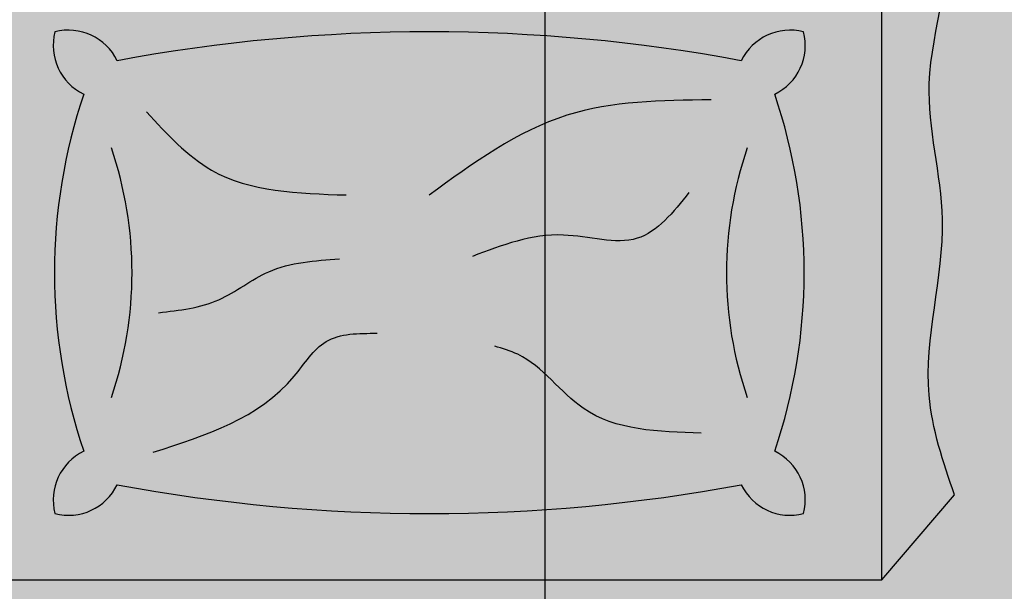
# Model space of a CAD drawing. Units: inches. Extents: x 1704 to 6393, y -157 to 1172.
# Tile 34 of 122: x 2529 to 2563, y 112 to 131. Entities that reach past the tile are written whole.
import ezdxf

# ---------------------------------------------------------------- set-up
doc = ezdxf.new("R2010")
doc.units = ezdxf.units.IN
doc.header["$MEASUREMENT"] = 0
for name, color, linetype, lineweight in [('A-ANNO-DIMS', 7, 'Continuous', 13), ('A-FURN', 8, 'Continuous', 18), ('estofado', 7, 'Continuous', 25)]:
    doc.layers.add(name, color=color, linetype=linetype, lineweight=lineweight)
doc.layers.add('A-FLOR-PATT', color=7, linetype='Continuous', lineweight=13, true_color=0xf2f2f2)
doc.styles.get("Standard").update_dxf_attribs({"font": 'arial.ttf'})
doc.dimstyles.get("Standard").update_dxf_attribs({"dimtxt": 6, "dimasz": 2, "dimexe": 0.18, "dimexo": 0.0625, "dimgap": 0.09, "dimtad": 0, "dimtih": 1, "dimtoh": 1, "dimdec": 1, "dimzin": 0, "dimdsep": 46, "dimlunit": 3, "dimtxsty": 'Standard', "dimblk": 'ARCHTICK', "dimcen": 0.09, "dimadec": 0, "dimazin": 0, "dimtfac": 1, "dimtdec": 1, "dimtofl": 0, "dimtmove": 0, "dimatfit": 3, "dimfxl": 1, "dimtolj": 1, "dimtzin": 0, "dimarcsym": 0})

# ---------------------------------------------------------------- blocks, each defined once
blk = doc.blocks.new('Cama Box Regencia LOLA')
at = {"layer": 'estofado', "ltscale": 0.2}
h = blk.add_hatch(color=256, dxfattribs=at)
h.dxf.hatch_style = 1
h.set_gradient(color1=(240, 232, 219), color2=(213, 190, 154), one_color=1, tint=0.7200000286102295)
edge = h.paths.add_edge_path()
edge.add_line((-0.8000000000000682, -0.1548023628405417), (-0.863597199697665, -0.2293271111754507))
edge.add_spline(control_points=[(-0.8635971996977787, -0.2293271111754507), (-0.8537222782123308, -0.258285373872468), (-0.8269013755602826, -0.3369378214810581), (-0.8674912876567759, -0.4595932758330151), (-0.8253488717912205, -0.6001498518888299), (-0.8771423076391329, -0.7139760714239288), (-0.8243323781925938, -0.8129899320257435), (-0.885044987287756, -0.8716602542656914), (-0.879518062107536, -0.9542863467743244), (-0.8339551707063037, -1.008464155856984), (-0.8245672924600739, -1.059984630119799), (-0.8208601923470268, -1.104655887174089), (-0.8073908324747662, -1.131238421004809), (-0.7999999999999546, -1.145824641594799)], knot_values=[0, 0, 0, 0, 0.0901802310564388, 0.2449351320798513, 0.3646438241986237, 0.5132330690395209, 0.5950634960661151, 0.646820388242338, 0.740988272125753, 0.8098674202588053, 0.8551784313864677, 0.8950360916221496, 0.9434986994854018, 0.9434986994854018, 0.9434986994854018, 0.9434986994854018], degree=3, periodic=0)
edge.add_line((-0.7999999999999546, -1.145824641594856), (-0.7999999999999546, -0.9571831923306604))
edge.add_spline(control_points=[(-0.8000000000001818, -0.9571831923294098), (-0.8003674620557603, -0.9560020588672273), (-0.8014778173377408, -0.9524330433489467), (-0.799534669348418, -0.9460450666617248), (-0.7963405736333016, -0.9382358308520792), (-0.7944188048602429, -0.9289040147384638), (-0.7953122817383474, -0.9190683391483389), (-0.7985341887020923, -0.9137677522519994), (-0.7999999999999546, -0.911356242470788)], knot_values=[0, 0, 0, 0, 0.0036609130031785, 0.0110621328900358, 0.0190316076023675, 0.0292873612819121, 0.0393286152452009, 0.0477100398955968, 0.0477100398955968, 0.0477100398955968, 0.0477100398955968], degree=3, periodic=0)
edge.add_line((-0.8000000000000682, -0.9113562424705037), (-0.7999999999999546, -0.8573491405791173))
edge.add_spline(control_points=[(-0.7999999999999546, -0.8573491405791173), (-0.8011509914009592, -0.8570771933481751), (-0.804102924754261, -0.8563797336621519), (-0.8039036519178353, -0.8498286502876908), (-0.8010279369466388, -0.8413595542568258), (-0.805623441450507, -0.8302818657685406), (-0.801318481758244, -0.8238273834048186), (-0.7999999999999546, -0.8218505664625013)], knot_values=[0, 0, 0, 0, 0.0032305881034183, 0.0082854491905874, 0.015951437769388, 0.0315866871777379, 0.0384893971878813, 0.0384893971878813, 0.0384893971878813, 0.0384893971878813], degree=3, periodic=0)
edge.add_line((-0.7999999999999546, -0.821850566462558), (-0.7999999999999546, -0.7800193173444541))
edge.add_spline(control_points=[(-0.7999999999999546, -0.7800193173443404), (-0.7985416092056994, -0.7788853679199974), (-0.7956241855360986, -0.7766169698310819), (-0.7929439183725436, -0.7707329795046576), (-0.7969680334608711, -0.7644035258254576), (-0.7912681985083055, -0.7566015403456845), (-0.7963938877088595, -0.7483952775559715), (-0.798936373489596, -0.7431699116222604), (-0.799999999999841, -0.7409839258539251)], knot_values=[0, 0, 0, 0, 0.0055481279082489, 0.0110986984731684, 0.0174746050947868, 0.0251556172852474, 0.035519246289823, 0.0429729849735991, 0.0429729849735991, 0.0429729849735991, 0.0429729849735991], degree=3, periodic=0)
edge.add_line((-0.7999999999999546, -0.740983925853584), (-0.8000000000000682, -0.1548023628405417))
h = blk.add_hatch(color=256, dxfattribs=at)
h.dxf.hatch_style = 1
h.set_gradient(color1=(240, 232, 219), color2=(213, 190, 154), one_color=1, tint=0.7200000286102295, name='CURVED')
edge = h.paths.add_edge_path()
edge.add_spline(control_points=[(0.343533776195045, -0.8455058148597345), (0.2879313990920309, -0.8167160606696484), (0.2054770794474052, -0.7744470032542381), (0.0954193394759386, -0.7742416952675626), (-0.0885363502328574, -0.7276964167006668), (0.2428192566063672, -0.7672518992321216), (0.345087521536243, -0.8076697826234067), (0.3825206986321063, -0.8228555492498799)], knot_values=[0.0056315103357428, 0.0056315103357428, 0.0056315103357428, 0.0056315103357428, 0.1860138916206105, 0.2660015162584448, 0.3570871810327863, 0.5963901805690979, 0.739731738908988, 0.739731738908988, 0.739731738908988, 0.739731738908988], degree=3, periodic=0)
edge.add_spline(control_points=[(0.3825206986325611, -0.8228555492497662), (0.3974221570828149, -0.8135511441712424), (0.4121061736600496, -0.8037181558521524), (0.4266849906532571, -0.7937075488799225)], knot_values=[1.358237767273279, 1.358237767273279, 1.358237767273279, 1.358237767273279, 1.409915662372559, 1.409915662372559, 1.409915662372559, 1.409915662372559], degree=3, periodic=0)
edge.add_spline(control_points=[(0.4266849905698109, -0.7937075489369932), (0.3998777739682282, -0.7821381809783361), (0.3476761897024971, -0.7634757898491671), (0.2670618099601825, -0.7565375622627358), (0.0835725072796549, -0.7192994417154637), (0.288524529784695, -0.7446405493717521), (0.4247448861246994, -0.7759943071475277), (0.4449816270193879, -0.7810438091316882)], knot_values=[0.1043639306803623, 0.1043639306803623, 0.1043639306803623, 0.1043639306803623, 0.1896363068641149, 0.2696239315019491, 0.3607095962762907, 0.6000125958126024, 0.6446217338078729, 0.6446217338078729, 0.6446217338078729, 0.6446217338078729], degree=3, periodic=0)
edge.add_spline(control_points=[(0.4449816270197289, -0.7810438091316882), (0.5029779388527232, -0.7406836481117695), (0.5966687145296419, -0.6736247633211292), (0.7071737530245628, -0.6656573253703187), (0.7517012483331201, -0.6672238302253392)], knot_values=[1.43159032281798, 1.43159032281798, 1.43159032281798, 1.43159032281798, 1.63814180148235, 1.770695287284994, 1.770695287284994, 1.770695287284994, 1.770695287284994], degree=3, periodic=0)
edge.add_arc((0.7481853615017826, -0.767162003811734), 0.0999999999999888, 58.7920033978138, 87.98512997550938, ccw=False)
edge.add_line((0.8000000000000682, -0.6816328085782289), (0.8000000000000682, -0.154802362840428))
edge.add_line((0.8000000000000682, -0.154802362840428), (-0.7999999999999546, -0.154802362840428))
edge.add_line((-0.7999999999999546, -0.154802362840428), (-0.8000000000000682, -0.7409839258539819))
edge.add_spline(control_points=[(-0.799999999999841, -0.7409839258539251), (-0.7846451382113174, -0.74846387981205), (-0.7568940913494089, -0.7651582159765554), (-0.7559936909002545, -0.8096905380045313), (-0.7049413305308008, -0.8142555457367848), (-0.7013836936888538, -0.8139988647640733)], knot_values=[0.0122267587020837, 0.0122267587020837, 0.0122267587020837, 0.0122267587020837, 0.0594720782072034, 0.1062176618094138, 0.134458043575382, 0.134458043575382, 0.134458043575382, 0.134458043575382], degree=3, periodic=0)
edge.add_spline(control_points=[(-0.7013836936890812, -0.8139988647637892), (-0.6428309483887916, -0.8132695376718857), (-0.532520673001045, -0.8118955240036598), (-0.2390712668254764, -0.6717984706609172), (-0.3892411364554391, -0.7557901092520752), (-0.4591093260188473, -0.8070101468627512), (-0.5571511178645779, -0.795652750469742), (-0.608497950975675, -0.8409486634728295), (-0.6632498050151981, -0.8266781836207997), (-0.6991149398675134, -0.8254126024436914), (-0.719552182989446, -0.8246914287938125)], knot_values=[0, 0, 0, 0, 0.2187005959148062, 0.4120203559900679, 0.4786136596093368, 0.6046444033330721, 0.6969970394608519, 0.7456449795902803, 0.7925683322559657, 0.8547274388453192, 0.8547274388453192, 0.8547274388453192, 0.8547274388453192], degree=3, periodic=0)
edge.add_spline(control_points=[(-0.7195521829781911, -0.824691428792164), (-0.7293124663336812, -0.8248308281530967), (-0.7545977292818407, -0.8216412233076653), (-0.7742556984202338, -0.794819860189591), (-0.7939222919129634, -0.7820064600295497), (-0.799999999999841, -0.7800193173443404)], knot_values=[0.1564883932805935, 0.1564883932805935, 0.1564883932805935, 0.1564883932805935, 0.184397548386913, 0.2313764834161266, 0.2505984550882281, 0.2505984550882281, 0.2505984550882281, 0.2505984550882281], degree=3, periodic=0)
edge.add_line((-0.8000000000000682, -0.7800193173444541), (-0.7999999999999546, -0.8218505664627286))
edge.add_spline(control_points=[(-0.7999999999999546, -0.8218505664625013), (-0.7938082505512511, -0.8290217081292894), (-0.7673857405620766, -0.8512914803976059), (-0.7619109683460011, -0.8661369353891359), (-0.6555700939965164, -0.8510070218793543), (-0.7139793977868294, -0.8637526923380391), (-0.7379026254519659, -0.8623504601624176), (-0.7688129786438367, -0.8813042143888196), (-0.7854260296310259, -0.8561610219318254), (-0.7961930533253962, -0.8566031243811949), (-0.7999999999999546, -0.8573491405791173)], knot_values=[0.0595743221876141, 0.0595743221876141, 0.0595743221876141, 0.0595743221876141, 0.08075289116965, 0.1037414994169835, 0.1697200936249022, 0.1760361327243865, 0.2071371586311508, 0.2404744334261798, 0.2623408547027293, 0.2736604507987723, 0.2736604507987723, 0.2736604507987723, 0.2736604507987723], degree=3, periodic=0)
edge.add_line((-0.7999999999999546, -0.8573491405791173), (-0.8000000000000682, -0.9113562424721521))
edge.add_spline(control_points=[(-0.8000000000000682, -0.9113562424720385), (-0.7937204054647964, -0.9077594990848183), (-0.7710343135782978, -0.8978798065321029), (-0.7213062468074442, -0.9144666877443228), (-0.6268586829058905, -0.862430497409548), (-0.6896594748232019, -0.9045634991654196), (-0.7483442493064559, -0.9189273406958591), (-0.7835301183422417, -0.922920432793262), (-0.7896301351460125, -0.9477657000142585), (-0.7975786973822779, -0.955260590410262), (-0.8000000000001818, -0.9571831923294098)], knot_values=[0.0138560263374175, 0.0138560263374175, 0.0138560263374175, 0.0138560263374175, 0.0348737775836104, 0.0888666909546002, 0.1078792274429341, 0.1267378491223226, 0.1587140219647659, 0.1937574699451985, 0.2174867851300671, 0.2267221218327879, 0.2267221218327879, 0.2267221218327879, 0.2267221218327879], degree=3, periodic=0)
edge.add_line((-0.7999999999999546, -0.957183192329296), (-0.7999999999999546, -1.145824641594742))
edge.add_spline(control_points=[(-0.8000000000002955, -1.145824641594913), (-0.7271039467997298, -1.094596787649038), (-0.4885706936571524, -0.9465888221489535), (-0.0701640902225336, -0.9707493165000187), (0.237911901821235, -0.902164522332157), (0.3435337762145991, -0.845505814843193)], knot_values=[0.1168958193629841, 0.1168958193629841, 0.1168958193629841, 0.1168958193629841, 0.3797203297758731, 0.9577018633805092, 1.31379338443587, 1.31379338443587, 1.31379338443587, 1.31379338443587], degree=3, periodic=0)
h.paths.add_polyline_path([(-0.6766340706021765, -0.6101327540145576, -0.3575266660906883), (-0.7312746368313583, -0.6354535276154252, -0.3575266660894137), (-0.7059538632299791, -0.5808129613865844, -0.1647847126465284), (-0.7059538632300928, -0.2676124402649407, -0.3575266660890756), (-0.7312746368312446, -0.2129718740360431, -0.3575266660908716), (-0.6766340706020629, -0.2382926476369676, -0.0925607043966334), (-0.1295169377724505, -0.2382926476369107, -0.3575266660898965), (-0.0748763715433825, -0.2129718740360431, -0.3575266660894428), (-0.1001971451446479, -0.2676124402649407, -0.1647847126465285), (-0.1001971451445343, -0.5808129613865844, -0.3575266660890756), (-0.0748763715433825, -0.6354535276154821, -0.3575266660898962), (-0.1295169377724505, -0.6101327540146145, -0.0925607043966531)], flags=16)
h.paths.add_polyline_path([(0.0748763715433825, -0.6354535276157094, -0.3575266660910266), (0.1001971451446479, -0.5808129613865844, -0.1647847126465284), (0.1001971451445343, -0.2676124402649407, -0.3575266660890757), (0.0748763715433825, -0.2129718740360431, -0.3575266660898962), (0.1295169377724505, -0.2382926476369107, -0.0925607043966334), (0.6766340706020629, -0.2382926476369676, -0.3575266660908718), (0.7312746368312446, -0.2129718740360431, -0.3575266660894425), (0.7059538632299791, -0.2676124402649407, -0.1647847126465283), (0.7059538632300928, -0.5808129613865844, -0.3575266660890756), (0.7312746368312446, -0.6354535276154821, -0.3575266660908716), (0.6766340706020629, -0.6101327540145576, -0.0925607043966335), (0.1295169377724505, -0.6101327540146145, -0.3575266660906303)], flags=16)
h = blk.add_hatch(color=256, dxfattribs=at)
h.dxf.hatch_style = 1
h.set_gradient(color1=(106, 82, 42), color2=(160, 123, 64), one_color=1, tint=0.4399999976158142, name='CURVED')
h.paths.add_polyline_path([(-0.1001971451445343, -0.2676124402650544, 0.3575266660914516), (-0.0748763715433825, -0.2129718740358157, 0.3575266660906303), (-0.1295169377724505, -0.2382926476369107, 0.0925607043966334), (-0.6766340706020629, -0.2382926476369676, 0.3575266660908717), (-0.7312746368312446, -0.2129718740360431, 0.3575266660886796), (-0.7059538632300928, -0.2676124402648838, 0.1647847126464969), (-0.7059538632300928, -0.5808129613864708, 0.3575266660910845), (-0.731274636831131, -0.6354535276157094, 0.3575266660898384), (-0.6766340706021765, -0.6101327540146145, 0.0925607043966531), (-0.1295169377724505, -0.6101327540146145, 0.3575266660898962), (-0.0748763715433825, -0.6354535276154821, 0.3575266660883126), (-0.1001971451444206, -0.5808129613866413, 0.164784712646497)])
blk.add_line((-0.7999999999999546, -0.154802362840428), (-0.8635971996977787, -0.2293271111754507), dxfattribs=at)
blk.add_lwpolyline([(0.8000000000000682, -0.6816328085741361), (0.8000000000000682, -0.154802362840428), (-0.7999999999999546, -0.154802362840428), (-0.7999999999999546, -0.7409839258540956)], dxfattribs=at)
for centre, radius, start, end in [((-0.6852907786285414, -0.2248498560688859), 0.047493175008304, 165.516646303857, 244.209945069049), ((-0.7193966547980608, -0.2589557322385758), 0.047493175008304, 25.79005493108792, 104.4833536962803), ((-0.4030755041873136, -1.703357436968531), 1.490385562932656, 79.42346065608027, 100.5765393439127), ((-0.0867543535765663, -0.2589557322385758), 0.047493175008304, 75.51664630371964, 154.2099450689121), ((-0.120860229745972, -0.2248498560688859), 0.047493175008304, 295.790054930951, 14.48335369614292), ((-0.243690300061985, -0.4242127008258194), 0.4880688921049917, 161.2852469077218, 198.7147530922607), ((-0.562460708312642, -0.4242127008258194), 0.4880688921049917, 341.2852469077393, 18.71475309227822), ((-1.002461858008359, -0.4242127008257626), 0.3387897965243698, 341.1598423418016, 18.84015765820971), ((0.19631084963396, -0.4242127008257626), 0.3387897965243698, 161.1598423417902, 198.8401576581983), ((-0.6852907786285414, -0.6235755455826393), 0.047493175008304, 115.790054930951, 194.4833536961429), ((-0.120860229745972, -0.6235755455826393), 0.047493175008304, 345.516646303857, 64.20994506904903), ((-0.7193966547980608, -0.5894696694129494), 0.047493175008304, 255.5166463037197, 334.2099450689121), ((-0.4030755041873136, 0.8549320353169491), 1.490385562932656, 259.4234606560872, 280.5765393439197), ((-0.0867543535765663, -0.5894696694129494), 0.047493175008304, 205.7900549310879, 284.4833536962804)]:
    blk.add_arc(centre, radius, start, end, dxfattribs=at)
for points, knots in [([(-0.8635971996977787, -0.2293271111754507), (-0.8537222782123597, -0.2582853738724713), (-0.8269013755602529, -0.3369378214810687), (-0.8674912876567628, -0.459593275832977), (-0.8253488717912105, -0.6001498518888299), (-0.8771423076387755, -0.7139760714238776), (-0.824332378192706, -0.8129899320257793), (-0.8850449872876955, -0.8716602542656513), (-0.8795180621076731, -0.9542863467744586), (-0.8339551707061605, -1.008464155856879), (-0.8245672924602526, -1.059984630119836), (-0.820860192346876, -1.104655887174075), (-0.8073908324747767, -1.131238421004865), (-0.7999999999999546, -1.145824641594799)], [0, 0, 0, 0, 0.0901802310564388, 0.2449351320798513, 0.3646438241986237, 0.5132330690395209, 0.5950634960661151, 0.646820388242338, 0.740988272125753, 0.8098674202588053, 0.8551784313864677, 0.8950360916221496, 0.9434986994854018, 0.9434986994854018, 0.9434986994854018, 0.9434986994854018]), ([(-0.1609929429250769, -0.2668120520876869), (-0.207361296664481, -0.2816189425177519), (-0.2673465842344797, -0.3007741531050562), (-0.3100088172549912, -0.3711986237053177), (-0.3410959220547441, -0.371113456673647), (-0.3573768361287648, -0.371068853062809)], [0, 0, 0, 0, 0.1404794637529129, 0.1817338842404631, 0.2270973195475621, 0.2270973195475621, 0.2270973195475621, 0.2270973195475621]), ([(-0.641547568925148, -0.2836087781224137), (-0.6039704843628328, -0.2846768301159754), (-0.539944686002343, -0.2864966328594507), (-0.4983244357833337, -0.3487001107148991), (-0.4673537235191868, -0.3577134183149331), (-0.460449429265168, -0.3597227530484019)], [0, 0, 0, 0, 0.1057518620258909, 0.1801855432155129, 0.2015394496060149, 0.2015394496060149, 0.2015394496060149, 0.2015394496060149]), ([(-0.1657269282603693, -0.3891622340328808), (-0.1839821155447316, -0.3912290170364152), (-0.2191851220416109, -0.3952145677934529), (-0.2641538569791404, -0.4324302667024541), (-0.3028411853428648, -0.4348886966416372), (-0.3243911361614664, -0.4362581125853354)], [0, 0, 0, 0, 0.0540396012867365, 0.1042090889319622, 0.1672963371706364, 0.1672963371706364, 0.1672963371706364, 0.1672963371706364]), ([(-0.630774277431101, -0.4946666993113809), (-0.6169895699779718, -0.4772535648042688), (-0.5885015945383536, -0.441266950663047), (-0.5131074616321869, -0.4662255111125919), (-0.4667910825139399, -0.4484404284426592), (-0.4408934738504513, -0.4384959742387196)], [0, 0, 0, 0, 0.0606588350328579, 0.1253597443752535, 0.2074214353097695, 0.2074214353097695, 0.2074214353097695, 0.2074214353097695]), ([(-0.6501439432536245, -0.5758072434303472), (-0.6067249420939599, -0.5753127958675333), (-0.5155219215609228, -0.5742741927209986), (-0.4416129136043037, -0.5203678897559305), (-0.402889750189047, -0.4921247481343585)], [0, 0, 0, 0, 0.1270530108164939, 0.2668789710677518, 0.2668789710677518, 0.2668789710677518, 0.2668789710677518]), ([(-0.1552772464440295, -0.5652394970176715), (-0.1730924483668451, -0.5457941389807961), (-0.2188221854511549, -0.4958799637506091), (-0.2880058022633399, -0.4937226941133118), (-0.3302371516485891, -0.4924058446629829)], [0, 0, 0, 0, 0.0765478869158952, 0.1964903209174588, 0.1964903209174588, 0.1964903209174588, 0.1964903209174588])]:
    blk.add_open_spline(points, degree=3, knots=knots, dxfattribs=at)
blk = doc.blocks.new('_ArchTick')
at = {"color": 0, "linetype": 'ByBlock', "const_width": 0.15}
blk.add_lwpolyline([(-0.5, -0.5), (0.5, 0.5)], dxfattribs=at)
blk = doc.blocks.new('*D93')
at = {"layer": 'A-ANNO-DIMS', "color": 0, "lineweight": -2, "transparency": 16777216}
for p, q in [((2605.286074000001, 895.2129740000005), (1829.697551000002, 895.2129740000003)), ((1829.877551000002, 895.2129740000003), (1829.877551000002, 495.8664119263302)), ((1829.877551000002, 90.2129739999999), (1829.877551000002, 489.5595360736699)), ((2605.286074000001, 90.21297400000003), (1829.697551000002, 90.2129739999999))]:
    blk.add_line(p, q, dxfattribs=at)
at = {"layer": 'Defpoints', "color": 0, "lineweight": -3, "transparency": 16777216}
for p in [(2605.348574000001, 895.2129740000005), (1829.877551000002, 90.2129739999999), (2605.348574000001, 90.21297400000003)]:
    blk.add_point(p, dxfattribs=at)
at = {"layer": 'A-ANNO-DIMS', "color": 0, "lineweight": -2, "transparency": 16777216, "xscale": 2, "yscale": 2, "zscale": 2}
for p, rotation in [((1829.877551000002, 895.2129740000003), 90), ((1829.877551000002, 90.2129739999999), 270)]:
    blk.add_blockref('_ArchTick', p, dxfattribs=dict(at, rotation=rotation))
at = {"layer": 'A-ANNO-DIMS', "color": 0, "transparency": 16777216, "insert": (1829.877551000001, 492.7129739999994), "char_height": 6, "attachment_point": 5}
blk.add_mtext('\\A1;805', dxfattribs=at)
blk = doc.blocks.new('*D105')
at = {"layer": 'A-ANNO-DIMS', "color": 0, "lineweight": -2, "transparency": 16777216}
for p, q in [((2451.737975, 615.150474), (2451.737975, -64.9670259999999)), ((2547.348574, 615.150474), (2547.348574, -64.9670259999999)), ((2451.737975, -64.787026), (2489.908936164393, -64.787026)), ((2547.348574, -64.787026), (2509.177612835607, -64.787026))]:
    blk.add_line(p, q, dxfattribs=at)
at = {"layer": 'Defpoints', "color": 0, "lineweight": -3, "transparency": 16777216}
for p in [(2451.737975, 615.212974), (2547.348574, 615.212974), (2547.348574, -64.787026)]:
    blk.add_point(p, dxfattribs=at)
at = {"layer": 'A-ANNO-DIMS', "color": 0, "lineweight": -2, "transparency": 16777216, "xscale": 2, "yscale": 2, "zscale": 2, "rotation": 180}
blk.add_blockref('_ArchTick', (2451.737975, -64.787026), dxfattribs=at)
at = {"layer": 'A-ANNO-DIMS', "color": 0, "lineweight": -2, "transparency": 16777216, "xscale": 2, "yscale": 2, "zscale": 2}
blk.add_blockref('_ArchTick', (2547.348574, -64.787026), dxfattribs=at)
at = {"layer": 'A-ANNO-DIMS', "color": 0, "transparency": 16777216, "insert": (2499.5432745, -64.787026), "char_height": 6, "attachment_point": 5}
blk.add_mtext('\\A1;95.61', dxfattribs=at)

msp = doc.modelspace()

# ---------------------------------------------------------------- hatches: boundary and pattern name
at = {"layer": 'A-FLOR-PATT', "transparency": 33554528}
h = msp.add_hatch(color=256, dxfattribs=at)
h.dxf.hatch_style = 1
h.paths.add_polyline_path([(2325.348574056059, 863.2129735309796), (2325.348574056059, 887.2129735309796), (2263.348574056059, 887.2129735309796), (2167.348574056059, 887.2129735309794), (2081.348574056061, 887.2129735309792), (2081.348574056061, 719.2129735309785), (2277.348574056059, 719.2129735309787), (2277.348574056059, 711.2129735309788), (2277.348574056059, 372.212973530979), (2349.348574056059, 372.212973530979), (2381.348574056059, 372.2129735309789), (2381.348574056059, 364.2129735309789), (2353.348574056059, 364.2129735309789), (2353.348574056059, 270.2129735309788), (2381.348574056059, 270.2129735309788), (2381.348574056059, 266.2129735309788), (2357.348574056059, 266.2129735309788), (2357.348574056059, 98.21297353097884), (2381.348574056059, 98.21297353097897), (2385.181056550604, 98.21297353097884), (2386.482186711948, 98.21297353097884), (2424.21496140017, 98.21297353097884), (2425.516091561514, 98.21297353097884), (2429.348574056059, 98.21297353097897), (2597.348574056059, 98.21297353097884), (2597.348574056059, 146.2129735309788), (2597.348574056059, 218.2129735309788), (2597.348574056059, 266.2129735309788), (2423.348574056059, 266.2129735309788), (2423.348574056059, 270.2129735309788), (2473.348574056059, 270.2129735309788), (2473.348574056059, 294.2129735309789), (2477.348574056059, 294.2129735309789), (2477.348574056059, 270.2129735309788), (2547.348574056059, 270.2129735309788), (2547.348574056059, 364.2129735309788), (2477.348574056059, 364.2129735309788), (2477.348574056059, 318.2129735309788), (2473.348574056059, 318.2129735309787), (2473.348574056059, 364.2129735309789), (2423.348574056059, 364.2129735309788), (2423.348574056059, 372.2129735309788), (2469.348574056059, 372.2129735309788), (2469.348574056059, 459.2129735309789), (2469.348574056059, 538.2129735309788), (2350.348574056059, 538.2129735309788), (2350.348574056059, 565.7129735309788), (2358.348574056059, 565.7129735309788), (2358.348574056059, 545.2129735309788), (2420.348574056059, 545.2129735309788), (2420.348574056059, 610.2129735309788), (2358.348574056059, 610.2129735309788), (2358.348574056059, 589.7129735309788), (2350.348574056059, 589.7129735309788), (2350.348574056059, 615.2129735309788), (2425.348574056059, 615.2129735309788), (2425.348574056059, 607.2129735309788), (2425.348574056059, 546.2129735309788), (2469.348574056059, 546.2129735309788), (2514.34857405606, 546.212973530979), (2514.34857405606, 607.2129735309788), (2449.348574056059, 607.2129735309788), (2449.348574056059, 615.2129735309788), (2451.737974987759, 615.2129735309788), (2451.737974987759, 659.2129735309788), (2427.737974987759, 659.2129735309788), (2427.737974987759, 665.2129735309788), (2367.737974987758, 665.2129735309788), (2367.737974987758, 667.2129735309788), (2367.737974987758, 711.2129735309788), (2325.348574056059, 711.2129735309788), (2325.348574056059, 719.2129735309785), (2325.348574056059, 755.2129735309787), (2325.348574056059, 763.2129735309788)])
h.paths.add_polyline_path([(2233.85817000392, 822.532660166629, -0.1872470486944155), (2233.85817000392, 809.1396667958562), (2231.697030374885, 808.8044951349628, 0.0848927708004382), (2233.130501812631, 814.4858417746204), (2230.423974436808, 814.4858417746204, -0.1042581087707907), (2228.553363812687, 808.3129425443484), (2217.750790159711, 807.1555239386723, -0.2222222222222219), (2217.750790159711, 824.5168030238124), (2228.553363812687, 823.3593844181363, -0.1042581087707933), (2230.423974436808, 817.1864851878643), (2233.130501812631, 817.1864851878643, 0.08489277080044), (2231.697030374885, 822.8678318275219)], flags=16)
h.paths.add_polyline_path([(2213.621360876743, 833.1974425663823), (2213.621360876743, 798.4748843961024), (2156.047684459484, 798.4748843961034), (2156.047684459485, 833.1974425663813)], flags=16)
h.paths.add_polyline_path([(2203.931929661768, 848.0987249710489), (2205.089348267444, 837.2961513180724, -0.2222222222222264), (2187.728069182304, 837.2961513180724), (2188.88548778798, 848.0987249710485, -0.104258108770792), (2195.058387018252, 849.9693355951691), (2195.058387018252, 852.6758629709927, 0.084892770800438), (2189.377040378595, 851.2423915332469), (2189.712212039488, 853.4035311622828, -0.1872470486944166), (2203.105205410261, 853.4035311622828), (2203.440377071154, 851.2423915332469, 0.084892770800438), (2197.759030431496, 852.6758629709927), (2197.759030431496, 849.9693355951691, -0.1042581087707896)], flags=16)
h.paths.add_polyline_path([(2181.940976153924, 837.2961513180726, -0.2222222222222323), (2164.579697068783, 837.2961513180724), (2165.73711567446, 848.0987249710487, -0.1042581087707905), (2171.910014904732, 849.9693355951691), (2171.910014904732, 852.6758629709927, 0.0848927708004445), (2166.228668265074, 851.2423915332469), (2166.563839925967, 853.403531162283, -0.1872470486944096), (2179.95683329674, 853.4035311622828), (2180.292004957633, 851.2423915332465, 0.0848927708004458), (2174.610658317976, 852.6758629709927), (2174.610658317976, 849.9693355951691, -0.104258108770801), (2180.783557548248, 848.0987249710482)], flags=16)
h.paths.add_polyline_path([(2205.089348267444, 794.376175644412), (2203.931929661768, 783.5736019914364, -0.1042581087707934), (2197.759030431496, 781.7029913673155), (2197.759030431496, 778.9964639914921, 0.084892770800439), (2203.440377071154, 780.4299354292382), (2203.105205410261, 778.2687958002022, -0.1872470486944172), (2189.712212039488, 778.2687958002018), (2189.377040378595, 780.4299354292377, 0.0848927708004369), (2195.058387018252, 778.9964639914919), (2195.058387018252, 781.7029913673153, -0.1042581087707904), (2188.88548778798, 783.5736019914358), (2187.728069182304, 794.3761756444126, -0.2222222222222231)], flags=16)
h.paths.add_polyline_path([(2181.940976153924, 794.376175644412), (2180.783557548248, 783.5736019914364, -0.1042581087708008), (2174.610658317976, 781.7029913673153), (2174.610658317976, 778.9964639914921, 0.0848927708004458), (2180.292004957633, 780.4299354292382), (2179.95683329674, 778.268795800202, -0.1872470486944096), (2166.563839925967, 778.2687958002018), (2166.228668265074, 780.4299354292378, 0.0848927708004446), (2171.910014904732, 778.9964639914919), (2171.910014904732, 781.7029913673153, -0.1042581087707904), (2165.73711567446, 783.5736019914358), (2164.579697068783, 794.3761756444123, -0.2222222222222294)], flags=16)
h.paths.add_polyline_path([(2151.918255176517, 807.1555239386723), (2141.115681523541, 808.3129425443484, -0.1042581087707911), (2139.24507089942, 814.4858417746204), (2136.538543523597, 814.4858417746204, 0.08489277080044), (2137.972014961343, 808.8044951349626), (2135.810875332307, 809.1396667958562, -0.1872470486944109), (2135.810875332307, 822.5326601666285), (2137.972014961343, 822.8678318275221, 0.0848927708004416), (2136.538543523597, 817.1864851878643), (2139.24507089942, 817.1864851878643, -0.104258108770793), (2141.115681523541, 823.3593844181363), (2151.918255176517, 824.5168030238124, -0.2222222222222205)], flags=16)
h.paths.add_polyline_path([(2357.868011454448, 363.4102250290031), (2358.813881560335, 363.4102250290031, 0.7537604849588476)], flags=16)
h.paths.add_polyline_path([(2372.241054283868, 363.1167008961685), (2372.248110816919, 363.1167008961685), (2372.248110816919, 363.3425764997267), (2371.30224071103, 363.3425764997267), (2371.30224071103, 363.1392706554335, -1.360391292333951)], flags=16)
h.paths.add_polyline_path([(2371.309297244092, 272.7157694655011), (2371.30224071103, 272.7157694655011), (2371.30224071103, 272.4898938619428), (2372.248110816919, 272.4898938619428), (2372.248110816919, 272.6931997062759, -1.360391292393621)], flags=16)
h.paths.add_polyline_path([(2357.875067987504, 272.7157694655011), (2357.868011454452, 272.7157694655011), (2357.868011454452, 272.4898938619428), (2358.813881560341, 272.4898938619428), (2358.813881560341, 272.6931997062361, -1.360391292333948)], flags=16)
h.paths.add_polyline_path([(2353.768696905258, 363.0736921025416), (2376.347425366111, 363.0736921025416), (2376.347425366111, 272.7587782591281), (2353.768696905258, 272.7587782591281)], flags=16)
h.paths.add_polyline_path([(2354.772195947961, 362.0701930598379), (2375.343926323407, 362.0701930598379), (2375.343926323407, 273.7622773018316), (2354.772195947961, 273.7622773018318)], flags=0)
h.paths.add_polyline_path([(2357.868011454452, 363.3425764997267), (2358.813881560341, 363.3425764997266), (2358.813881560341, 363.1167008961684), (2357.868011454452, 363.1167008961684)], flags=16)
h.paths.add_polyline_path([(2359.287941640134, 359.1843485433627), (2359.287941640134, 360.0631949744305), (2370.828180631237, 360.0631949744362), (2370.828180631237, 359.1843485433769), (2374.332057422314, 359.1843485433812), (2374.332057422312, 358.4635369582513), (2372.835178716611, 358.4635369582524), (2372.835178716611, 357.5410357047662), (2374.332057422314, 357.5410357047678), (2374.332057422312, 356.8202241196381), (2372.835178716611, 356.820224119639), (2372.835178716611, 355.897722866153), (2374.332057422314, 355.8977228661546), (2374.332057422312, 355.1769112810248), (2372.835178716611, 355.1769112810259), (2372.835178716611, 354.2544100275397), (2374.332057422334, 354.2544100275415), (2374.332057422331, 353.5335984424117), (2372.835178716631, 353.5335984424126), (2372.835178716631, 352.6110971889265), (2374.332057422334, 352.6110971889282), (2374.332057422331, 351.8902856037984), (2372.835178716631, 351.8902856037993), (2372.835178716631, 350.9677843503132), (2374.332057422334, 350.967784350315), (2374.332057422331, 350.2469727651852), (2372.835178716631, 350.2469727651861), (2372.835178716631, 349.3244715117), (2374.332057422334, 349.3244715117017), (2374.332057422331, 348.603659926572), (2372.835178716631, 348.6036599265729), (2372.835178716631, 347.6811586730868), (2374.332057422334, 347.6811586730886), (2374.332057422331, 346.9603470879587), (2372.835178716631, 346.9603470879598), (2372.835178716631, 346.0378458344735), (2374.332057422334, 346.0378458344753), (2374.332057422331, 345.3170342493456), (2372.835178716631, 345.3170342493465), (2372.835178716631, 344.3945329958605), (2374.332057422334, 344.3945329958621), (2374.332057422331, 343.6737214107324), (2372.835178716631, 343.6737214107334), (2372.835178716631, 342.751220157247), (2374.332057422334, 342.7512201572489), (2374.332057422331, 342.0304085721191), (2372.835178716631, 342.03040857212), (2372.835178716631, 341.1079073186338), (2374.332057422334, 341.1079073186356), (2374.332057422331, 340.3870957335057), (2372.835178716631, 340.3870957335066), (2372.835178716631, 339.4645944800207), (2374.332057422334, 339.4645944800223), (2374.332057422331, 338.7437828948924), (2372.835178716648, 338.7437828948933), (2372.835178716648, 337.8212816414076), (2374.332057422334, 337.8212816414093), (2374.332057422331, 337.1004700562794), (2372.835178716648, 337.1004700562803), (2372.835178716648, 336.1779688027942), (2374.332057422334, 336.1779688027961), (2374.332057422331, 335.4571572176662), (2372.835178716648, 335.4571572176673), (2372.835178716648, 334.5346559641809), (2374.332057422334, 334.5346559641828), (2374.332057422331, 333.8138443790529), (2372.835178716648, 333.8138443790539), (2372.835178716648, 332.8913431255679), (2374.332057422334, 332.8913431255696), (2374.332057422331, 332.1705315404397), (2372.835178716648, 332.1705315404406), (2372.835178716648, 331.2480302869545), (2374.332057422334, 331.2480302869563), (2374.332057422331, 330.5272187018265), (2372.835178716648, 330.5272187018273), (2372.835178716648, 329.6047174483413), (2374.332057422334, 329.6047174483431), (2374.332057422331, 328.8839058632133), (2372.835178716648, 328.8839058632143), (2372.835178716648, 327.9614046097282), (2374.332057422334, 327.9614046097298), (2374.332057422331, 327.2405930246), (2372.835178716648, 327.2405930246009), (2372.835178716648, 326.3180917711149), (2374.332057422334, 326.3180917711167), (2374.332057422331, 325.5972801859869), (2372.835178716648, 325.5972801859877), (2372.835178716648, 324.6747789325016), (2374.332057422334, 324.6747789325034), (2374.332057422331, 323.9539673473736), (2372.835178716648, 323.9539673473746), (2372.835178716648, 323.0314660938884), (2374.332057422334, 323.0314660938901), (2374.332057422331, 322.3106545087603), (2372.835178716648, 322.3106545087613), (2372.835178716648, 321.3881532552753), (2374.332057422334, 321.388153255277), (2374.332057422331, 320.6673416701471), (2372.835178716648, 320.6673416701481), (2372.835178716648, 319.7448404166621), (2374.332057422334, 319.7448404166638), (2374.332057422331, 319.0240288315339), (2372.835178716648, 319.0240288315348), (2372.835178716648, 318.1015275780487), (2374.332057422334, 318.1015275780504), (2374.332057422331, 317.3807159929205), (2372.835178716648, 317.3807159929214), (2372.835178716648, 316.4582147394357), (2374.332057422334, 316.4582147394373), (2374.332057422331, 315.7374031543073), (2372.835178716648, 315.7374031543084), (2372.835178716648, 314.8149019008223), (2374.332057422334, 314.8149019008241), (2374.332057422331, 314.0940903156943), (2372.835178716648, 314.0940903156952), (2372.835178716648, 313.171589062209), (2374.332057422334, 313.1715890622108), (2374.332057422331, 312.450777477081), (2372.835178716648, 312.4507774770819), (2372.835178716648, 311.5282762235959), (2374.332057422334, 311.5282762235977), (2374.332057422331, 310.8074646384678), (2372.835178716648, 310.8074646384687), (2372.835178716648, 309.8849633849827), (2374.332057422334, 309.8849633849844), (2374.332057422331, 309.1641517998546), (2372.835178716648, 309.1641517998555), (2372.835178716648, 308.2416505463693), (2374.332057422334, 308.2416505463712), (2374.332057422331, 307.5208389612412), (2372.835178716648, 307.5208389612421), (2372.835178716648, 306.5983377077562), (2374.332057422334, 306.598337707758), (2374.332057422331, 305.8775261226281), (2372.835178716648, 305.8775261226289), (2372.835178716648, 304.955024869143), (2374.332057422334, 304.9550248691447), (2374.332057422331, 304.2342132840149), (2372.835178716648, 304.2342132840158), (2372.835178716648, 303.3117120305298), (2374.332057422334, 303.3117120305316), (2374.332057422331, 302.5909004454018), (2372.835178716648, 302.5909004454027), (2372.835178716648, 301.6683991919165), (2374.332057422334, 301.6683991919183), (2374.332057422331, 300.9475876067885), (2372.835178716648, 300.9475876067894), (2372.835178716648, 300.0250863533033), (2374.332057422334, 300.025086353305), (2374.332057422331, 299.3042747681752), (2372.835178716648, 299.3042747681761), (2372.835178716648, 298.3817735146902), (2374.332057422334, 298.3817735146919), (2374.332057422331, 297.6609619295621), (2372.835178716648, 297.6609619295629), (2372.835178716648, 296.7384606760769), (2374.332057422334, 296.7384606760786), (2374.332057422331, 296.0176490909488), (2372.835178716648, 296.0176490909498), (2372.835178716648, 295.0951478374636), (2374.332057422334, 295.0951478374653), (2374.332057422331, 294.3743362523355), (2372.835178716648, 294.3743362523364), (2372.835178716648, 293.4518349988504), (2374.332057422334, 293.4518349988522), (2374.332057422331, 292.7310234137224), (2372.835178716648, 292.7310234137233), (2372.835178716648, 291.8085221602371), (2374.332057422334, 291.8085221602389), (2374.332057422331, 291.0877105751091), (2372.835178716648, 291.08771057511), (2372.835178716648, 290.165209321624), (2374.332057422334, 290.1652093216256), (2374.332057422331, 289.4443977364957), (2372.835178716648, 289.4443977364966), (2372.835178716648, 288.5218964830108), (2374.332057422334, 288.5218964830125), (2374.332057422331, 287.8010848978827), (2372.835178716648, 287.8010848978836), (2372.835178716648, 286.8785836443975), (2374.332057422334, 286.8785836443993), (2374.332057422331, 286.1577720592695), (2372.835178716648, 286.1577720592703), (2372.835178716648, 285.2352708057842), (2374.332057422334, 285.2352708057861), (2374.332057422331, 284.5144592206562), (2372.835178716648, 284.514459220657), (2372.835178716648, 283.5919579671712), (2374.332057422334, 283.5919579671728), (2374.332057422331, 282.871146382043), (2372.835178716648, 282.8711463820439), (2372.835178716648, 281.9486451285579), (2374.332057422334, 281.9486451285596), (2374.332057422331, 281.2278335434298), (2372.835178716648, 281.2278335434307), (2372.835178716648, 280.3053322899446), (2374.332057422334, 280.3053322899464), (2374.332057422331, 279.5845207048164), (2372.835178716648, 279.5845207048174), (2372.835178716648, 278.6620194513314), (2374.332057422334, 278.6620194513331), (2374.332057422331, 277.9412078662033), (2372.835178716648, 277.9412078662043), (2372.835178716648, 277.0187066127184), (2374.332057422334, 277.0187066127201), (2374.332057422331, 276.29789502759), (2370.828180631244, 276.2978950275922), (2370.828180631244, 275.7692753872335), (2359.287941640128, 275.7692753872392), (2359.287941640128, 276.2978950275993), (2355.784064849037, 276.2978950276015), (2355.784064849037, 277.0187066126971), (2357.280943554723, 277.0187066126989), (2357.280943554723, 277.9412078662137), (2355.784064849037, 277.9412078662145), (2355.784064849037, 278.6620194513103), (2357.280943554723, 278.6620194513122), (2357.280943554723, 279.5845207048271), (2355.784064849037, 279.584520704828), (2355.784064849037, 280.3053322899236), (2357.280943554723, 280.3053322899253), (2357.280943554723, 281.2278335434403), (2355.784064849037, 281.2278335434412), (2355.784064849037, 281.9486451285369), (2357.280943554723, 281.9486451285387), (2357.280943554723, 282.8711463820535), (2355.784064849037, 282.8711463820543), (2355.784064849037, 283.5919579671501), (2357.280943554723, 283.591957967152), (2357.280943554723, 284.5144592206668), (2355.784064849037, 284.5144592206676), (2355.784064849037, 285.2352708057632), (2357.280943554723, 285.2352708057651), (2357.280943554723, 286.1577720592801), (2355.784064849037, 286.1577720592809), (2355.784064849037, 286.8785836443766), (2357.280943554723, 286.8785836443784), (2357.280943554723, 287.8010848978931), (2355.784064849037, 287.8010848978941), (2355.784064849037, 288.5218964829895), (2357.280943554723, 288.5218964829913), (2357.280943554723, 289.4443977365064), (2355.784064849037, 289.4443977365072), (2355.784064849037, 290.1652093216029), (2357.280943554723, 290.1652093216047), (2357.280943554723, 291.0877105751197), (2355.784064849037, 291.0877105751206), (2355.784064849037, 291.8085221602161), (2357.280943554723, 291.8085221602179), (2357.280943554723, 292.7310234137328), (2355.784064849037, 292.7310234137337), (2355.784064849037, 293.4518349988293), (2357.280943554723, 293.451834998831), (2357.280943554723, 294.3743362523461), (2355.784064849037, 294.3743362523469), (2355.784064849037, 295.0951478374426), (2357.280943554723, 295.0951478374445), (2357.280943554723, 296.0176490909594), (2355.784064849037, 296.0176490909601), (2355.784064849037, 296.7384606760557), (2357.280943554723, 296.7384606760575), (2357.280943554723, 297.6609619295724), (2355.784064849037, 297.6609619295734), (2355.784064849037, 298.3817735146691), (2357.280943554723, 298.3817735146709), (2357.280943554723, 299.3042747681858), (2355.784064849037, 299.3042747681866), (2355.784064849037, 300.0250863532823), (2357.280943554723, 300.0250863532841), (2357.280943554723, 300.9475876067989), (2355.784064849037, 300.9475876067997), (2355.784064849037, 301.6683991918954), (2357.280943554723, 301.6683991918973), (2357.280943554723, 302.5909004454123), (2355.784064849037, 302.5909004454133), (2355.784064849037, 303.3117120305088), (2357.280943554723, 303.3117120305105), (2357.280943554723, 304.2342132840254), (2355.784064849037, 304.2342132840262), (2355.784064849037, 304.9550248691219), (2357.280943554723, 304.9550248691238), (2357.280943554723, 305.8775261226386), (2355.784064849037, 305.8775261226394), (2355.784064849037, 306.5983377077352), (2357.280943554723, 306.5983377077369), (2357.280943554723, 307.5208389612518), (2355.784064849037, 307.5208389612528), (2355.784064849037, 308.2416505463484), (2357.280943554723, 308.2416505463501), (2357.280943554723, 309.1641517998652), (2355.784064849037, 309.1641517998661), (2355.784064849037, 309.8849633849617), (2357.280943554723, 309.8849633849634), (2357.280943554723, 310.8074646384782), (2355.784064849037, 310.8074646384791), (2355.784064849037, 311.5282762235748), (2357.280943554723, 311.5282762235767), (2357.280943554723, 312.4507774770916), (2355.784064849037, 312.4507774770925), (2355.784064849037, 313.171589062188), (2357.280943554723, 313.1715890621898), (2357.280943554723, 314.0940903157049), (2355.784064849037, 314.0940903157058), (2355.784064849037, 314.8149019008013), (2357.280943554723, 314.8149019008032), (2357.280943554723, 315.7374031543179), (2355.784064849037, 315.7374031543187), (2355.784064849037, 316.4582147394146), (2357.280943554723, 316.4582147394165), (2357.280943554723, 317.3807159929311), (2355.784064849037, 317.3807159929321), (2355.784064849037, 318.1015275780277), (2357.280943554723, 318.1015275780295), (2357.280943554723, 319.0240288315445), (2355.784064849037, 319.0240288315454), (2355.784064849037, 319.744840416641), (2357.280943554723, 319.7448404166428), (2357.280943554723, 320.6673416701576), (2355.784064849037, 320.6673416701585), (2355.784064849037, 321.3881532552541), (2357.280943554723, 321.388153255256), (2357.280943554723, 322.3106545087708), (2355.784064849037, 322.3106545087718), (2355.784064849037, 323.0314660938674), (2357.280943554723, 323.0314660938692), (2357.280943554723, 323.9539673473843), (2355.784064849037, 323.9539673473851), (2355.784064849037, 324.6747789324806), (2357.280943554723, 324.6747789324824), (2357.280943554723, 325.5972801859974), (2355.784064849037, 325.5972801859983), (2355.784064849037, 326.3180917710939), (2357.280943554723, 326.3180917710958), (2357.280943554723, 327.2405930246105), (2355.784064849037, 327.2405930246113), (2355.784064849037, 327.9614046097071), (2357.280943554723, 327.961404609709), (2357.280943554723, 328.8839058632238), (2355.784064849037, 328.8839058632245), (2355.784064849037, 329.6047174483202), (2357.280943554723, 329.604717448322), (2357.280943554723, 330.527218701837), (2355.784064849037, 330.5272187018379), (2355.784064849037, 331.2480302869335), (2357.280943554723, 331.2480302869353), (2357.280943554723, 332.1705315404502), (2355.784064849037, 332.170531540451), (2355.784064849037, 332.8913431255468), (2357.280943554723, 332.8913431255486), (2357.280943554723, 333.8138443790634), (2355.784064849037, 333.8138443790642), (2355.784064849037, 334.5346559641599), (2357.280943554723, 334.5346559641618), (2357.280943554723, 335.4571572176767), (2355.784064849037, 335.4571572176776), (2355.784064849037, 336.1779688027732), (2357.280943554723, 336.177968802775), (2357.280943554723, 337.1004700562898), (2355.784064849037, 337.1004700562908), (2355.784064849037, 337.8212816413864), (2357.280943554723, 337.8212816413883), (2357.280943554723, 338.7437828949031), (2355.784064849037, 338.743782894904), (2355.784064849037, 339.4645944799996), (2357.280943554706, 339.4645944800013), (2357.280943554706, 340.3870957335163), (2355.784064849037, 340.3870957335173), (2355.784064849037, 341.1079073186129), (2357.280943554706, 341.1079073186146), (2357.280943554706, 342.0304085721296), (2355.784064849037, 342.0304085721304), (2355.784064849037, 342.7512201572262), (2357.280943554706, 342.751220157228), (2357.280943554706, 343.6737214107429), (2355.784064849037, 343.6737214107437), (2355.784064849037, 344.3945329958394), (2357.280943554706, 344.3945329958412), (2357.280943554706, 345.317034249356), (2355.784064849037, 345.3170342493569), (2355.784064849037, 346.0378458344526), (2357.280943554706, 346.0378458344544), (2357.280943554706, 346.9603470879692), (2355.784064849037, 346.9603470879701), (2355.784064849037, 347.6811586730658), (2357.280943554706, 347.6811586730677), (2357.280943554706, 348.6036599265824), (2355.784064849037, 348.6036599265833), (2355.784064849037, 349.324471511679), (2357.280943554706, 349.3244715116809), (2357.280943554706, 350.2469727651956), (2355.784064849037, 350.2469727651966), (2355.784064849037, 350.9677843502922), (2357.280943554706, 350.9677843502939), (2357.280943554706, 351.8902856038089), (2355.784064849037, 351.8902856038098), (2355.784064849037, 352.6110971889055), (2357.280943554706, 352.6110971889072), (2357.280943554706, 353.5335984424222), (2355.784064849037, 353.533598442423), (2355.784064849037, 354.2544100275187), (2357.280943554686, 354.2544100275204), (2357.280943554686, 355.1769112810354), (2355.784064849017, 355.1769112810362), (2355.784064849017, 355.897722866132), (2357.280943554686, 355.8977228661338), (2357.280943554686, 356.8202241196486), (2355.784064849017, 356.8202241196495), (2355.784064849017, 357.5410357047453), (2357.280943554686, 357.5410357047471), (2357.280943554686, 358.4635369582618), (2355.784064849017, 358.4635369582626), (2355.784064849017, 359.1843485433584)], flags=0)

# ---------------------------------------------------------------- block references
at = {"layer": 'A-FURN', "xscale": 39.22313671019584, "yscale": 39.22313671019584, "zscale": 39.22313671019584, "rotation": 180}
msp.add_blockref('Cama Box Regencia LOLA', (2527.569415053021, 106.0625493409584), dxfattribs=at)

# ---------------------------------------------------------------- dimensions: what is measured, and where the dimension line sits
at = {"layer": 'A-ANNO-DIMS'}
dim = msp.add_linear_dim(base=(1829.877551000002, 90.2129739999999), p1=(2605.348574000001, 895.212974), p2=(2605.348574000001, 90.21297399999999), angle=90, dimstyle='Standard', override={"dimdec": 0, "dimlfac": 1, "dimrnd": 0, "dimzin": 0, "dimdsep": 46, "dimlunit": 2}, dxfattribs=at)
dim.commit()
dim.dimension.update_dxf_attribs({"geometry": '*D93', "text_midpoint": (1829.877551000001, 492.7129739999994)})
dim = msp.add_linear_dim(base=(2547.348574, -64.787026), p1=(2451.737975, 615.212974), p2=(2547.348574, 615.212974), dimstyle='Standard', override={"dimdec": 2, "dimlfac": 1, "dimrnd": 0, "dimzin": 0, "dimdsep": 46, "dimlunit": 2}, dxfattribs=at)
dim.commit()
dim.dimension.update_dxf_attribs({"geometry": '*D105', "text_midpoint": (2499.5432745, -64.787026)})

doc.saveas('drawing.dxf')
